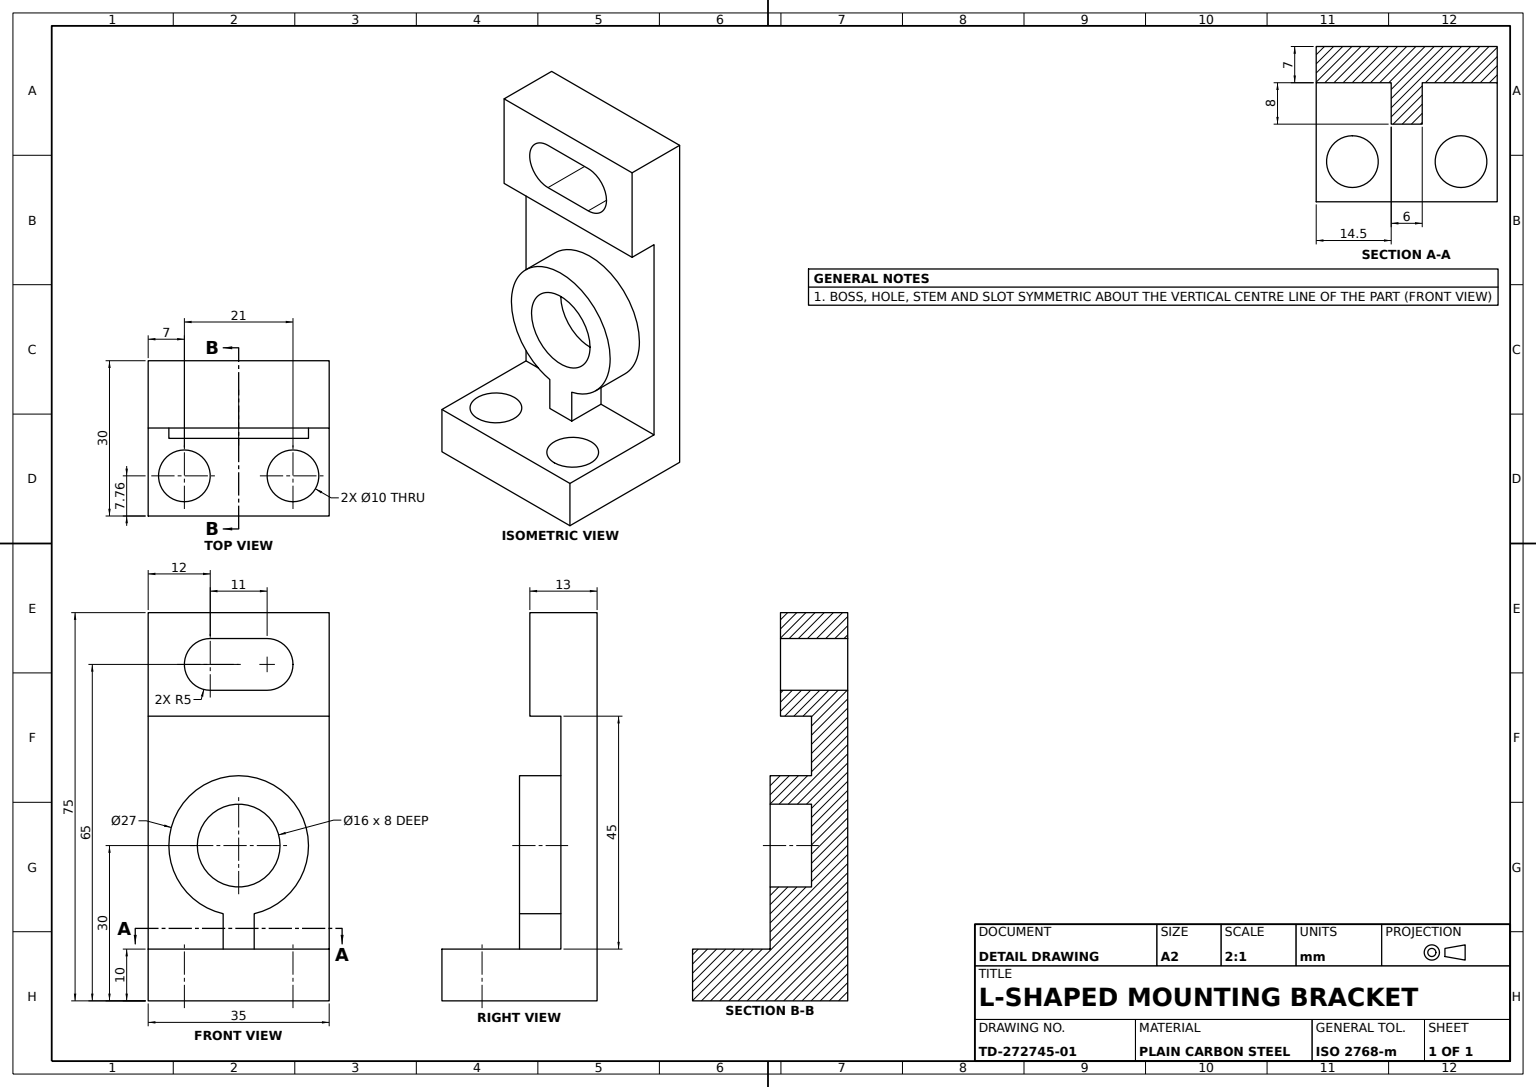
from build123d import *

# Parameters (mm, degrees)
L_BRACKET_BODY_DEPTH         = 17.5
UPRIGHT_SLOT_DEPTH           = 35
CORNER_SUPPORT_BOSS_SKETCH_R = 8
CORNER_SUPPORT_BOSS_DEPTH    = 8
DOWEL_HOLE_10_D              = 10


with BuildPart() as part:
    # L-Bracket Profile Sketch → L-Bracket Body (new, symmetric)
    with BuildSketch(Plane(origin=(0, 0, 0), x_dir=(0, 0, -1), z_dir=(1, 0, 0))):
        Polygon((0, 0), (30, 0), (30, 10), (7, 10), (7, 55), (13, 55), (13, 75), (0, 75), align=None)
    extrude(amount=L_BRACKET_BODY_DEPTH, both=True)

    # Upright Slot Sketch → Upright Slot (cut)
    with BuildSketch(Plane(origin=(0, 0, -13), x_dir=(-1, 0, 0), z_dir=(0, 0, -1))):
        with BuildLine():
            Line((-5.5, 70), (5.5, 70))
            ThreePointArc((5.5, 70), (10.5, 65), (5.5, 60))
            Line((5.5, 60), (-5.5, 60))
            ThreePointArc((-5.5, 60), (-10.5, 65), (-5.5, 70))
        make_face()
    extrude(amount=-UPRIGHT_SLOT_DEPTH, mode=Mode.SUBTRACT)

    # Corner Support Boss Sketch → Corner Support Boss (add)
    with BuildSketch(Plane(origin=(0, 0, -7), x_dir=(-1, 0, 0), z_dir=(0, 0, -1))):
        with BuildLine():
            Line((-3, 16.837553419), (-3, 10))
            Line((-3, 10), (3, 10))
            Line((3, 10), (3, 16.837553419))
            ThreePointArc((3, 16.837553419), (0, 43.5), (-3, 16.837553419))
        make_face()
        with Locations((0, 30)):
            Circle(CORNER_SUPPORT_BOSS_SKETCH_R, mode=Mode.SUBTRACT)
    extrude(amount=CORNER_SUPPORT_BOSS_DEPTH)

    # Dowel Hole Ø10 (through all)
    with Locations(Plane(origin=(0, 10, 0), x_dir=(1, 0, 0), z_dir=(0, 1, 0))):
        with Locations((-10.5, 22.240638775), (10.5, 22.240638775)):
            Hole(DOWEL_HOLE_10_D / 2)


solid = part.part
